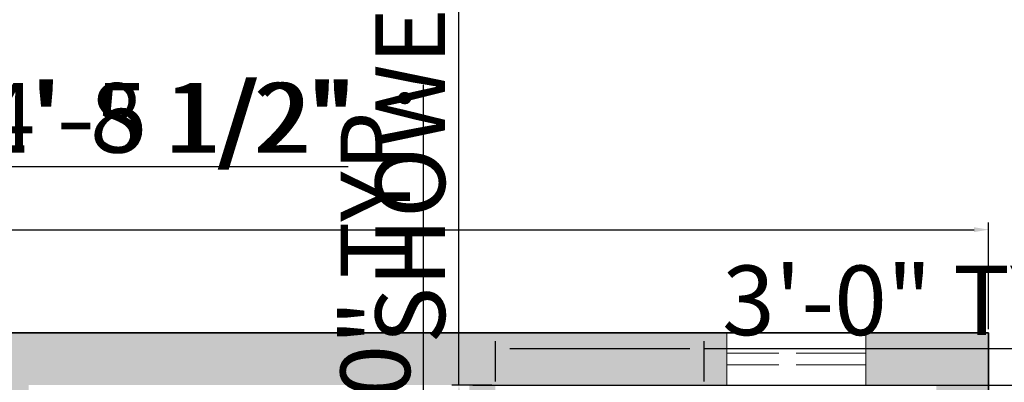
# Model space of a CAD drawing. Units: millimetres. Extents: x 542930 to 543750, y 628093 to 628738.
# Tile 11 of 14: x 543333 to 543502, y 628581 to 628644. Entities that reach past the tile are written whole.
import ezdxf

# ---------------------------------------------------------------- set-up
doc = ezdxf.new("R2010")
doc.units = ezdxf.units.MM
doc.linetypes.add('ACAD_ISO02W100', pattern=[15, 12, -3])
for name, color, linetype, lineweight in [('A-ANNO-DIMS', 2, 'Continuous', 18), ('A-GLAZ-HIDN', 70, 'ACAD_ISO02W100', 18), ('A-WALL', 7, 'Continuous', 35), ('WINDOW', 70, 'Continuous', 18)]:
    doc.layers.add(name, color=color, linetype=linetype, lineweight=lineweight)
doc.layers.add('A-WALL-PATT', color=251, linetype='Continuous', lineweight=13, true_color=0x636466)
doc.styles.get("Standard").update_dxf_attribs({"font": 'arial.ttf'})
doc.dimstyles.new('ISO-25', dxfattribs={"dimtxt": 12, "dimasz": 2.5, "dimexe": 1.25, "dimexo": 0.625, "dimtad": 1, "dimdec": 0, "dimlunit": 3, "dimtxsty": 'Standard', "dimcen": 2.5, "dimadec": 0, "dimazin": 0, "dimtfac": 1, "dimtdec": 0, "dimtmove": 0, "dimatfit": 3, "dimfxl": 1, "dimarcsym": 0})

# ---------------------------------------------------------------- blocks, each defined once
blk = doc.blocks.new('*D19')
at = {"layer": 'A-ANNO-DIMS', "color": 0, "lineweight": -2, "transparency": 16777216}
for p, q in [((542983.67, 628590.45), (542983.67, 628608.87)), ((543499.67, 628590.45), (543499.67, 628608.87)), ((542986.17, 628607.62), (543497.17, 628607.62))]:
    blk.add_line(p, q, dxfattribs=at)
at = {"layer": 'A-ANNO-DIMS', "color": 0, "transparency": 16777216}
for points in [[(542986.17, 628608.04), (542986.17, 628607.2), (542983.67, 628607.62)], [(543497.17, 628608.04), (543497.17, 628607.2), (543499.67, 628607.62)]]:
    blk.add_solid(points, dxfattribs=at)
at = {"layer": 'Defpoints', "color": 0, "transparency": 16777216}
for p in [(543499.67, 628607.62), (542983.67, 628589.83), (543499.67, 628589.83)]:
    blk.add_point(p, dxfattribs=at)
at = {"layer": 'A-ANNO-DIMS', "color": 0, "transparency": 16777216, "insert": (543241.67, 628614.38), "char_height": 12, "attachment_point": 5}
blk.add_mtext("43'", dxfattribs=at)
blk = doc.blocks.new('*D53')
at = {"layer": 'A-ANNO-DIMS', "color": 0, "lineweight": -2, "transparency": 16777216}
for p, q in [((543408.37, 628580.83), (543408.37, 628737.76)), ((543414.04, 628580.83), (543407.12, 628580.83)), ((543408.37, 628541.33), (543408.37, 628578.33)), ((543414.04, 628538.83), (543407.12, 628538.83))]:
    blk.add_line(p, q, dxfattribs=at)
at = {"layer": 'A-ANNO-DIMS', "color": 0, "transparency": 16777216}
for points in [[(543407.95, 628578.33), (543408.78, 628578.33), (543408.37, 628580.83)], [(543407.95, 628541.33), (543408.78, 628541.33), (543408.37, 628538.83)]]:
    blk.add_solid(points, dxfattribs=at)
at = {"layer": 'Defpoints', "color": 0, "transparency": 16777216}
for p in [(543408.37, 628580.83), (543414.67, 628580.83), (543414.67, 628538.83)]:
    blk.add_point(p, dxfattribs=at)
at = {"layer": 'A-ANNO-DIMS', "color": 0, "transparency": 16777216, "insert": (543401.53, 628660.54), "char_height": 12, "attachment_point": 5, "rotation": 90}
blk.add_mtext('SHOWER 3\'-6" TYP.', dxfattribs=at)
blk = doc.blocks.new('*D54')
at = {"layer": 'A-ANNO-DIMS', "color": 0, "lineweight": -2, "transparency": 16777216}
for p, q in [((543414.67, 628581.45), (543414.67, 628588.38)), ((543450.67, 628581.45), (543450.67, 628588.38)), ((543417.17, 628587.13), (543448.17, 628587.13)), ((543450.67, 628587.13), (543527.55, 628587.13))]:
    blk.add_line(p, q, dxfattribs=at)
at = {"layer": 'A-ANNO-DIMS', "color": 0, "transparency": 16777216}
for points in [[(543417.17, 628587.54), (543417.17, 628586.71), (543414.67, 628587.13)], [(543448.17, 628587.54), (543448.17, 628586.71), (543450.67, 628587.13)]]:
    blk.add_solid(points, dxfattribs=at)
at = {"layer": 'Defpoints', "color": 0, "transparency": 16777216}
for p in [(543450.67, 628587.13), (543414.67, 628580.83), (543450.67, 628580.83)]:
    blk.add_point(p, dxfattribs=at)
at = {"layer": 'A-ANNO-DIMS', "color": 0, "transparency": 16777216, "insert": (543490.36, 628593.88), "char_height": 12, "attachment_point": 5}
blk.add_mtext('3\'-0" TYP.', dxfattribs=at)
blk = doc.blocks.new('*D58')
at = {"layer": 'A-ANNO-DIMS', "color": 0, "lineweight": -2, "transparency": 16777216}
for p, q in [((543402.27, 628556.83), (543402.27, 628632.59)), ((543399.29, 628556.83), (543403.52, 628556.83)), ((543402.27, 628547.33), (543402.27, 628554.33)), ((543399.29, 628544.83), (543403.52, 628544.83))]:
    blk.add_line(p, q, dxfattribs=at)
at = {"layer": 'A-ANNO-DIMS', "color": 0, "transparency": 16777216}
for points in [[(543401.85, 628554.33), (543402.68, 628554.33), (543402.27, 628556.83)], [(543401.85, 628547.33), (543402.68, 628547.33), (543402.27, 628544.83)]]:
    blk.add_solid(points, dxfattribs=at)
at = {"layer": 'Defpoints', "color": 0, "transparency": 16777216}
for p in [(543398.67, 628556.83), (543402.27, 628556.83), (543398.67, 628544.83)]:
    blk.add_point(p, dxfattribs=at)
at = {"layer": 'A-ANNO-DIMS', "color": 0, "transparency": 16777216, "insert": (543395.51, 628595.96), "char_height": 12, "attachment_point": 5, "rotation": 90}
blk.add_mtext('1\'-0" TYP.', dxfattribs=at)
blk = doc.blocks.new('*D69')
at = {"layer": 'A-ANNO-DIMS', "color": 0, "lineweight": -2, "transparency": 16777216}
for p, q in [((543271.67, 628584.95), (543271.67, 628619.78)), ((543325.17, 628581.45), (543325.17, 628619.78)), ((543274.17, 628618.53), (543322.67, 628618.53)), ((543325.17, 628618.53), (543389.26, 628618.53))]:
    blk.add_line(p, q, dxfattribs=at)
at = {"layer": 'A-ANNO-DIMS', "color": 0, "transparency": 16777216}
for points in [[(543274.17, 628618.94), (543274.17, 628618.11), (543271.67, 628618.53)], [(543322.67, 628618.94), (543322.67, 628618.11), (543325.17, 628618.53)]]:
    blk.add_solid(points, dxfattribs=at)
at = {"layer": 'Defpoints', "color": 0, "transparency": 16777216}
for p in [(543325.17, 628618.53), (543271.67, 628584.33), (543325.17, 628580.83)]:
    blk.add_point(p, dxfattribs=at)
at = {"layer": 'A-ANNO-DIMS', "color": 0, "transparency": 16777216, "insert": (543358.46, 628625.36), "char_height": 12, "attachment_point": 5}
blk.add_mtext('4\'-5 1/2"', dxfattribs=at)
blk = doc.blocks.new('*D72')
at = {"layer": 'A-ANNO-DIMS', "color": 0, "lineweight": -2, "transparency": 16777216}
for p, q in [((543536.56, 628544.83), (543536.56, 628580.68)), ((543282.29, 628544.83), (543537.81, 628544.83)), ((543536.56, 628517.33), (543536.56, 628542.33)), ((543282.29, 628514.83), (543537.81, 628514.83))]:
    blk.add_line(p, q, dxfattribs=at)
at = {"layer": 'A-ANNO-DIMS', "color": 0, "transparency": 16777216}
for points in [[(543536.15, 628542.33), (543536.98, 628542.33), (543536.56, 628544.83)], [(543536.15, 628517.33), (543536.98, 628517.33), (543536.56, 628514.83)]]:
    blk.add_solid(points, dxfattribs=at)
at = {"layer": 'Defpoints', "color": 0, "transparency": 16777216}
for p in [(543281.67, 628544.83), (543536.56, 628544.83), (543281.67, 628514.83)]:
    blk.add_point(p, dxfattribs=at)
at = {"layer": 'A-ANNO-DIMS', "color": 0, "transparency": 16777216, "insert": (543529.81, 628564), "char_height": 12, "attachment_point": 5, "rotation": 90}
blk.add_mtext('2\'-6"', dxfattribs=at)
blk = doc.blocks.new('*D78')
at = {"layer": 'A-ANNO-DIMS', "color": 0, "lineweight": -2, "transparency": 16777216}
for p, q in [((543304.67, 628350.45), (543304.67, 628619.78)), ((543325.17, 628350.45), (543325.17, 628619.78)), ((543307.17, 628618.53), (543322.67, 628618.53)), ((543325.17, 628618.53), (543387.65, 628618.53))]:
    blk.add_line(p, q, dxfattribs=at)
at = {"layer": 'A-ANNO-DIMS', "color": 0, "transparency": 16777216}
for points in [[(543307.17, 628618.94), (543307.17, 628618.11), (543304.67, 628618.53)], [(543322.67, 628618.94), (543322.67, 628618.11), (543325.17, 628618.53)]]:
    blk.add_solid(points, dxfattribs=at)
at = {"layer": 'Defpoints', "color": 0, "transparency": 16777216}
for p in [(543325.17, 628618.53), (543304.67, 628349.83), (543325.17, 628349.83)]:
    blk.add_point(p, dxfattribs=at)
at = {"layer": 'A-ANNO-DIMS', "color": 0, "transparency": 16777216, "insert": (543357.66, 628625.36), "char_height": 12, "attachment_point": 5}
blk.add_mtext('1\'-8 1/2"', dxfattribs=at)
blk = doc.blocks.new('*D83')
at = {"layer": 'A-ANNO-DIMS', "color": 0, "lineweight": -2, "transparency": 16777216}
for p, q in [((543536.56, 628580.83), (543536.56, 628616.68)), ((543410.79, 628580.83), (543537.81, 628580.83)), ((543536.56, 628559.33), (543536.56, 628578.33)), ((543410.79, 628556.83), (543537.81, 628556.83))]:
    blk.add_line(p, q, dxfattribs=at)
at = {"layer": 'A-ANNO-DIMS', "color": 0, "transparency": 16777216}
for points in [[(543536.15, 628578.33), (543536.98, 628578.33), (543536.56, 628580.83)], [(543536.15, 628559.33), (543536.98, 628559.33), (543536.56, 628556.83)]]:
    blk.add_solid(points, dxfattribs=at)
at = {"layer": 'Defpoints', "color": 0, "transparency": 16777216}
for p in [(543410.17, 628580.83), (543536.56, 628580.83), (543410.17, 628556.83)]:
    blk.add_point(p, dxfattribs=at)
at = {"layer": 'A-ANNO-DIMS', "color": 0, "transparency": 16777216, "insert": (543529.81, 628600), "char_height": 12, "attachment_point": 5, "rotation": 90}
blk.add_mtext('2\'-0"', dxfattribs=at)

msp = doc.modelspace()

# ---------------------------------------------------------------- hatches: boundary and pattern name
at = {"layer": 'A-WALL-PATT'}
h = msp.add_hatch(color=256, dxfattribs=at)
h.dxf.hatch_style = 1
h.paths.add_polyline_path([(543454.53, 628589.83), (543271.67, 628589.83), (543271.67, 628580.83), (543325.17, 628580.83), (543325.17, 628475.36), (543334.17, 628475.36), (543334.17, 628481.83), (543370.17, 628481.83), (543370.17, 628490.83), (543334.17, 628490.83), (543334.17, 628580.83), (543410.17, 628580.83), (543410.17, 628524.86), (543414.67, 628524.86), (543414.67, 628580.83), (543454.53, 628580.83)])
h = msp.add_hatch(color=256, dxfattribs=at)
h.dxf.hatch_style = 1
h.paths.add_polyline_path([(543499.67, 628589.83), (543478.53, 628589.83), (543478.53, 628580.83), (543490.67, 628580.83), (543490.67, 628490.83), (543414.67, 628490.83), (543414.67, 628494.86), (543410.17, 628494.86), (543410.17, 628490.83), (543406.17, 628490.83), (543406.17, 628481.83), (543490.67, 628481.83), (543490.67, 628340.3), (543499.67, 628340.3)])

# ---------------------------------------------------------------- linework, layer by layer
at = {"layer": 'A-GLAZ-HIDN'}
for p, q in [((543478.53, 628586.33), (543454.53, 628586.33)), ((543478.53, 628584.33), (543454.53, 628584.33))]:
    msp.add_line(p, q, dxfattribs=at)
at = {"layer": 'A-WALL'}
msp.add_line((543499.67, 628589.83), (543499.67, 628253.83), dxfattribs=at)
msp.add_lwpolyline([(542983.67, 628589.83), (543499.67, 628589.83)], dxfattribs=at)
at = {"layer": 'WINDOW'}
for p, q in [((543454.53, 628589.83), (543454.53, 628580.83)), ((543478.53, 628589.83), (543478.53, 628580.83))]:
    msp.add_line(p, q, dxfattribs=at)

# ---------------------------------------------------------------- dimensions: what is measured, and where the dimension line sits
at = {"layer": 'A-ANNO-DIMS'}
for base, p1, p2, text, picture, middle in [((543408.37, 628580.83), (543414.67, 628538.83), (543414.67, 628580.83), 'SHOWER <> TYP.', '*D53', (543401.53, 628660.54)), ((543402.27, 628556.83), (543398.67, 628544.83), (543398.67, 628556.83), '<> TYP.', '*D58', (543395.51, 628595.96))]:
    dim = msp.add_linear_dim(base=base, p1=p1, p2=p2, angle=90, text=text, dimstyle='ISO-25', override={"dimdec": 1, "dimlfac": 1, "dimrnd": 0, "dimzin": 1, "dimdsep": 46, "dimlunit": 4, "dimfrac": 2}, dxfattribs=at)
    dim.commit()
    dim.dimension.update_dxf_attribs({"geometry": picture, "text_midpoint": middle})
for base, p1, p2, override, picture, middle in [((543325.17, 628618.53), (543271.67, 628584.33), (543325.17, 628580.83), {"dimdec": 1, "dimlfac": 1, "dimrnd": 0, "dimzin": 1, "dimdsep": 46, "dimlunit": 4, "dimfrac": 2}, '*D69', (543358.46, 628625.36)), ((543325.17, 628618.53), (543304.67, 628349.83), (543325.17, 628349.83), {"dimdec": 1, "dimlfac": 1, "dimrnd": 0, "dimzin": 1, "dimdsep": 46, "dimlunit": 4, "dimfrac": 2}, '*D78', (543357.66, 628625.36)), ((543499.67, 628607.62), (542983.67, 628589.83), (543499.67, 628589.83), {"dimclrd": 0, "dimclre": 0, "dimclrt": 0}, '*D19', (543241.67, 628614.38))]:
    dim = msp.add_linear_dim(base=base, p1=p1, p2=p2, dimstyle='ISO-25', override=override, dxfattribs=at)
    dim.commit()
    dim.dimension.update_dxf_attribs({"geometry": picture, "text_midpoint": middle})
for base, p1, p2, picture, middle in [((543536.56, 628580.83), (543410.17, 628556.83), (543410.17, 628580.83), '*D83', (543529.81, 628600)), ((543536.56, 628544.83), (543281.67, 628514.83), (543281.67, 628544.83), '*D72', (543529.81, 628564))]:
    dim = msp.add_linear_dim(base=base, p1=p1, p2=p2, angle=90, dimstyle='ISO-25', override={"dimdec": 1, "dimlfac": 1, "dimrnd": 0, "dimzin": 1, "dimdsep": 46, "dimlunit": 4, "dimfrac": 2}, dxfattribs=at)
    dim.commit()
    dim.dimension.update_dxf_attribs({"geometry": picture, "text_midpoint": middle})
dim = msp.add_linear_dim(base=(543450.67, 628587.13), p1=(543414.67, 628580.83), p2=(543450.67, 628580.83), text='<> TYP.', dimstyle='ISO-25', override={"dimdec": 1, "dimlfac": 1, "dimrnd": 0, "dimzin": 1, "dimdsep": 46, "dimlunit": 4, "dimfrac": 2}, dxfattribs=at)
dim.commit()
dim.dimension.update_dxf_attribs({"geometry": '*D54', "text_midpoint": (543490.36, 628593.88)})

doc.saveas('drawing.dxf')
